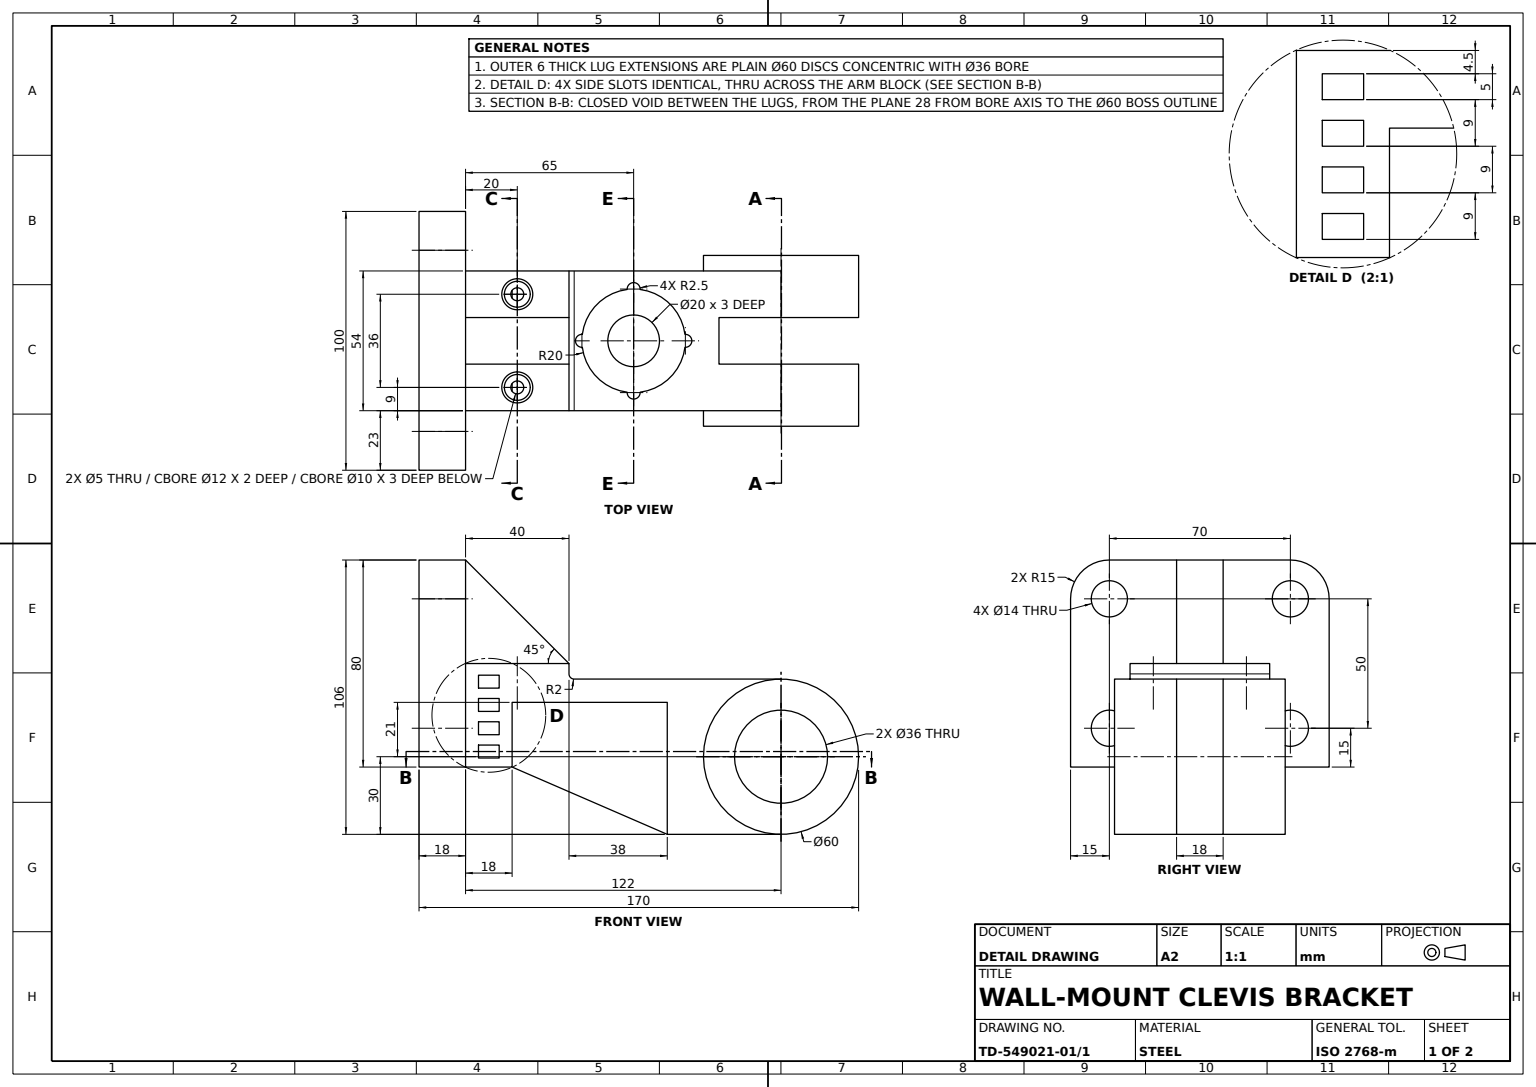
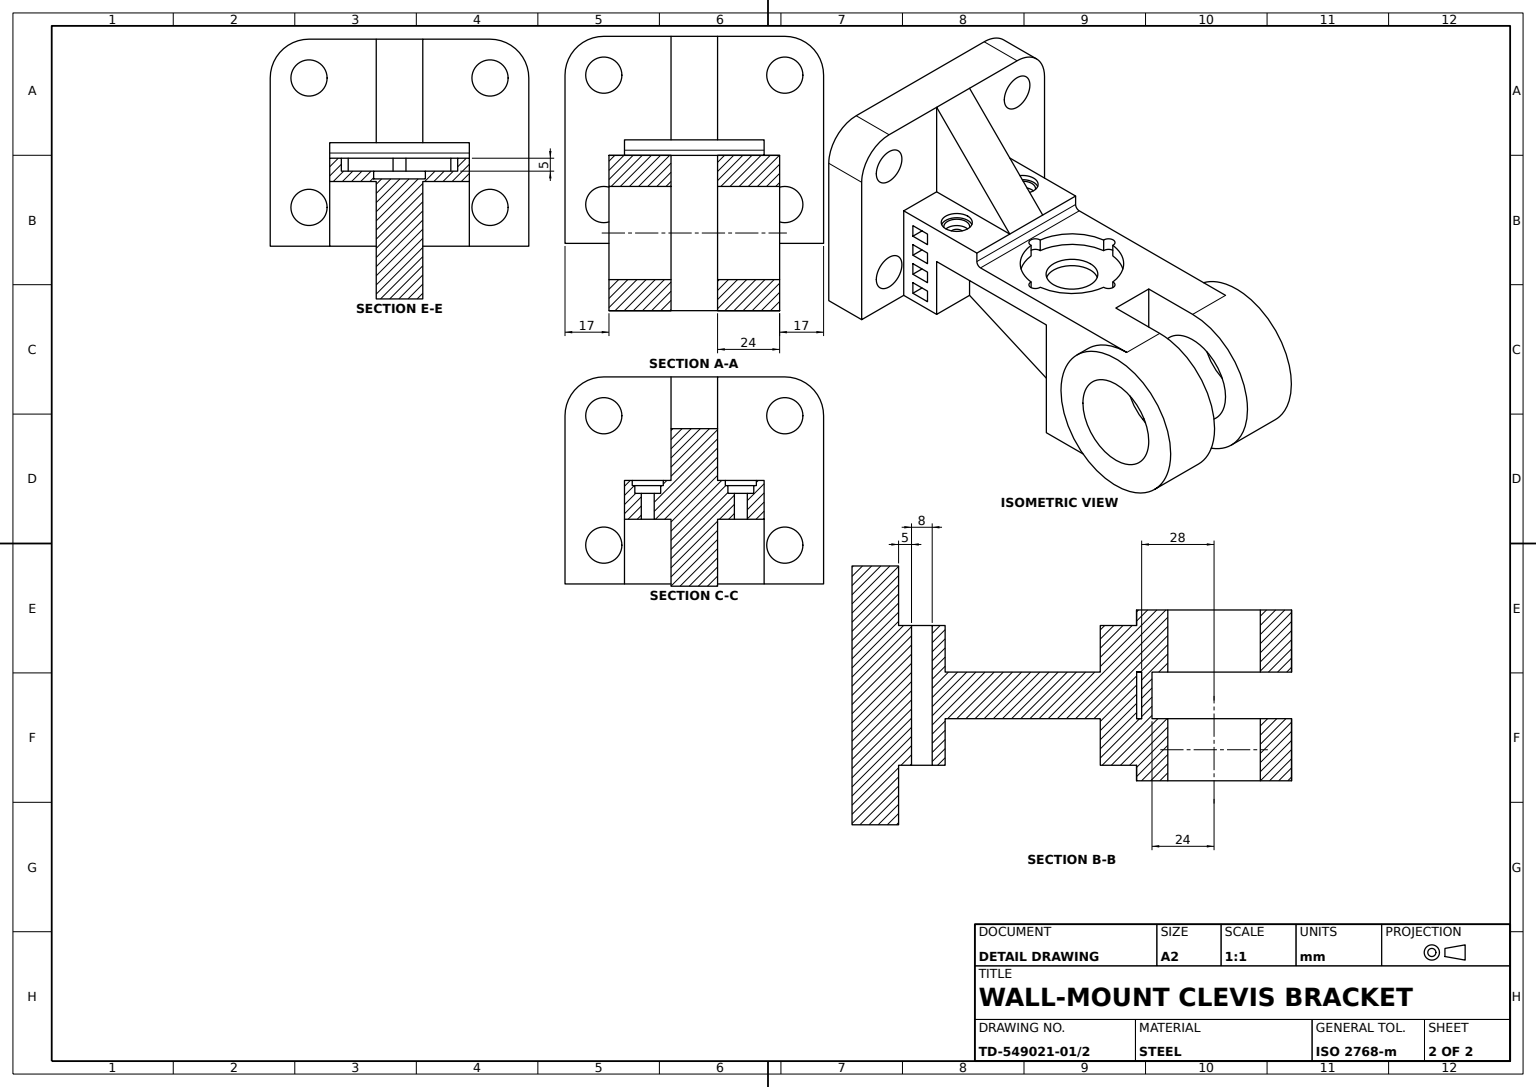
from build123d import *
from build123d.topology import SkipClean

# Parameters (mm, degrees)
MOUNTING_PLATE_SKETCH_R      = 9
MOUNTING_PLATE_DEPTH         = 18
ARM_BLOCK_SKETCH_W           = 18
ARM_BLOCK_SKETCH_H           = 54
ARM_BLOCK_DEPTH              = 40
PLATE_START                  = -18
PLATE_CORNER_BOSSES_SKETCH_R = 7
PLATE_CORNER_BOSSES_DEPTH    = 18
ARM_EXTENSION_SKETCH_W       = 40
ARM_EXTENSION_SKETCH_H       = 54
ARM_EXTENSION_DEPTH          = 15
UPPER_SUPPORT_RIB_REACH      = 88.394
UPPER_RIB_SKETCH_WALL_W      = 231.357431026
UPPER_RIB_SKETCH_WALL_H      = 18
CLEVIS_ARM_DEPTH             = 54
SKETCH7_4_R                  = 30
SKETCH7_4_R_2                = 18
CLEVIS_FACE_1_DEPTH          = 6
SKETCH7_5_R                  = 30
SKETCH7_5_R_2                = 18
CLEVIS_LUG_1_DEPTH           = 18
CLEVIS_START                 = -36
SKETCH7_6_R                  = 30
SKETCH7_6_R_2                = 18
CLEVIS_LUG_2_DEPTH           = 18
CLEVIS_START_2               = -54
SKETCH7_7_R                  = 30
SKETCH7_7_R_2                = 18
CLEVIS_FACE_2_DEPTH          = 6
CLEVIS_PIN_BORE_SKETCH_W     = 24
CLEVIS_PIN_BORE_SKETCH_H     = 18
CLEVIS_PIN_BORE_24_DEPTH     = 188.082869339
LOWER_SUPPORT_RIB_REACH      = 191.093
LOWER_RIB_SKETCH_WALL_W      = 445.576270742
LOWER_RIB_SKETCH_WALL_H      = 18
CLEVIS_WEB_PAD_SKETCH_W      = 4
CLEVIS_WEB_PAD_SKETCH_H      = 18
CLEVIS_WEB_PAD_DEPTH         = 60
ARM_BLOCK_HOLES_SKETCH_R     = 2.5
ARM_BLOCK_HOLES_DEPTH        = 15
COUNTERBORE_10_SKETCH_R      = 5
COUNTERBORE_10_DEPTH         = 5
SPOTFACE_12_SKETCH_R         = 6
SPOTFACE_12_DEPTH            = 2
SIDE_SLOTS_4X_SKETCH_W       = 8
SIDE_SLOTS_4X_SKETCH_H       = 5
SIDE_SLOTS_4X_DEPTH          = 198.952014387
KEYED_RECESS_SKETCH_R        = 10
KEYED_RECESS_DEPTH           = 5
RECESS_BORE_20_SKETCH_R      = 10
RECESS_BORE_20_DEPTH         = 8
ARM_EDGE_FILLET_R2_R         = 2


with BuildPart() as part:
    # Mounting Plate Sketch → Mounting Plate (new body)
    with BuildSketch(Plane(origin=(0, 0, 0), x_dir=(0, 0, -1), z_dir=(1, 0, 0))):
        with BuildLine():
            Line((-50, -40), (50, -40))
            Line((50, -40), (50, 25))
            ThreePointArc((50, 25), (45.606601718, 35.606601718), (35, 40))
            Line((35, 40), (-35, 40))
            ThreePointArc((-35, 40), (-45.606601718, 35.606601718), (-50, 25))
            Line((-50, 25), (-50, -40))
        make_face()
        with Locations((-35, 25)):
            Circle(MOUNTING_PLATE_SKETCH_R, mode=Mode.SUBTRACT)
        with Locations((35, 25)):
            Circle(MOUNTING_PLATE_SKETCH_R, mode=Mode.SUBTRACT)
        with Locations((-35, -25)):
            Circle(MOUNTING_PLATE_SKETCH_R, mode=Mode.SUBTRACT)
        with Locations((35, -25)):
            Circle(MOUNTING_PLATE_SKETCH_R, mode=Mode.SUBTRACT)
    extrude(amount=MOUNTING_PLATE_DEPTH)

    # Arm Block Sketch → Arm Block (add)
    with BuildSketch(Plane.XZ.offset(40)):
        with Locations((27, 0)):
            Rectangle(ARM_BLOCK_SKETCH_W, ARM_BLOCK_SKETCH_H)
    extrude(amount=-ARM_BLOCK_DEPTH)

    # Plate Corner Bosses Sketch → Plate Corner Bosses (add)
    with BuildSketch(Plane(origin=(18, 0, 0), x_dir=(0, 0, -1), z_dir=(1, 0, 0)).offset(PLATE_START)):
        with BuildLine():
            Line((-35, 40), (35, 40))
            ThreePointArc((35, 40), (45.606601718, 35.606601718), (50, 25))
            Line((50, 25), (50, -40))
            Line((50, -40), (-50, -40))
            Line((-50, -40), (-50, 25))
            ThreePointArc((-50, 25), (-45.606601718, 35.606601718), (-35, 40))
        make_face()
        with Locations((-35, 25)):
            Circle(PLATE_CORNER_BOSSES_SKETCH_R, mode=Mode.SUBTRACT)
        with Locations((35, 25)):
            Circle(PLATE_CORNER_BOSSES_SKETCH_R, mode=Mode.SUBTRACT)
        with Locations((35, -25)):
            Circle(PLATE_CORNER_BOSSES_SKETCH_R, mode=Mode.SUBTRACT)
        with Locations((-35, -25)):
            Circle(PLATE_CORNER_BOSSES_SKETCH_R, mode=Mode.SUBTRACT)
    extrude(amount=PLATE_CORNER_BOSSES_DEPTH)

    # Arm Extension Sketch → Arm Extension (add)
    with BuildSketch(Plane(origin=(0, 0, 0), x_dir=(1, 0, 0), z_dir=(0, 1, 0))):
        with Locations((38, 0)):
            Rectangle(ARM_EXTENSION_SKETCH_W, ARM_EXTENSION_SKETCH_H)
    extrude(amount=-ARM_EXTENSION_DEPTH)

    # Upper Rib Sketch wall → Upper Support Rib (add, up to next)
    with BuildSketch(Plane(origin=(38, 20, 0), x_dir=(0.707106781187, -0.707106781187, 0), z_dir=(0.707106781187, 0.707106781187, 0)), mode=Mode.PRIVATE) as upper_support_rib_sk1:
        Rectangle(UPPER_RIB_SKETCH_WALL_W, UPPER_RIB_SKETCH_WALL_H)
    upper_support_rib_tool1 = extrude(upper_support_rib_sk1.sketch, amount=-UPPER_SUPPORT_RIB_REACH, mode=Mode.PRIVATE) - part.part
    add(upper_support_rib_tool1.solids().sort_by_distance((38, 20, 0))[0])

    # Clevis Arm Profile Sketch → Clevis Arm (add)
    with BuildSketch(Plane.XY.offset(27)):
        with BuildLine():
            ThreePointArc((140, -66), (110, -36), (140, -6))
            Line((140, -6), (58, -6))
            Line((58, -6), (58, -15))
            Line((58, -15), (96, -15))
            Line((96, -15), (96, -66))
            Line((96, -66), (140, -66))
        make_face()
    extrude(amount=-CLEVIS_ARM_DEPTH)



with BuildPart() as body_2:
    # Sketch7_4 → Clevis Face 1 (new body)
    with BuildSketch(Plane.XY.offset(27)):
        with Locations((140, -36)):
            Circle(SKETCH7_4_R)
        with Locations((140, -36)):
            Circle(SKETCH7_4_R_2, mode=Mode.SUBTRACT)
    extrude(amount=CLEVIS_FACE_1_DEPTH)


with BuildPart() as part_1:
    with SkipClean():  # the faces are left unmerged after this step: merging them gives an invalid solid
        add(part.part)

        add(body_2.part)  # Clevis Lug 1 merges body 2
        # Sketch7_5 → Clevis Lug 1 (add)
        with BuildSketch(Plane.XY.offset(27)):
            with Locations((140, -36)):
                Circle(SKETCH7_5_R)
            with Locations((140, -36)):
                Circle(SKETCH7_5_R_2, mode=Mode.SUBTRACT)
        extrude(amount=-CLEVIS_LUG_1_DEPTH)

    # Sketch7_6 → Clevis Lug 2 (add)
    with SkipClean():  # the faces are left unmerged after this step: merging them gives an invalid solid
        with BuildSketch(Plane.XY.offset(27).offset(CLEVIS_START)):
            with Locations((140, -36)):
                Circle(SKETCH7_6_R)
            with Locations((140, -36)):
                Circle(SKETCH7_6_R_2, mode=Mode.SUBTRACT)
        extrude(amount=-CLEVIS_LUG_2_DEPTH)

    # Sketch7_7 → Clevis Face 2 (add)
    with SkipClean():  # the faces are left unmerged after this step: merging them gives an invalid solid
        with BuildSketch(Plane.XY.offset(27).offset(CLEVIS_START_2)):
            with Locations((140, -36)):
                Circle(SKETCH7_7_R)
            with Locations((140, -36)):
                Circle(SKETCH7_7_R_2, mode=Mode.SUBTRACT)
        extrude(amount=-CLEVIS_FACE_2_DEPTH)

    # Clevis Pin Bore Sketch → Clevis Pin Bore _24 (cut, through all)
    with SkipClean():  # the faces are left unmerged after this step: merging them gives an invalid solid
        with BuildSketch(Plane(origin=(0, -6, 0), x_dir=(1, 0, 0), z_dir=(0, 1, 0))):
            with Locations((128, 0)):
                Rectangle(CLEVIS_PIN_BORE_SKETCH_W, CLEVIS_PIN_BORE_SKETCH_H)
        extrude(amount=-CLEVIS_PIN_BORE_24_DEPTH, mode=Mode.SUBTRACT)

    # Lower Rib Sketch wall → Lower Support Rib (add, up to next)
    with BuildSketch(Plane(origin=(66, -53, 0), x_dir=(0.91755562531, -0.397607437634, 0), z_dir=(0.397607437634, 0.91755562531, 0)), mode=Mode.PRIVATE) as lower_support_rib_sk1:
        Rectangle(LOWER_RIB_SKETCH_WALL_W, LOWER_RIB_SKETCH_WALL_H)
    lower_support_rib_tool1 = extrude(lower_support_rib_sk1.sketch, amount=LOWER_SUPPORT_RIB_REACH, mode=Mode.PRIVATE) - part_1.part
    add(lower_support_rib_tool1.solids().sort_by_distance((66, -53, 0))[0])

    # Clevis Web Pad Sketch → Clevis Web Pad (add)
    with SkipClean():  # the faces are left unmerged after this step: merging them gives an invalid solid
        with BuildSketch(Plane(origin=(0, -6, 0), x_dir=(1, 0, 0), z_dir=(0, 1, 0))):
            with Locations((114, 0)):
                Rectangle(CLEVIS_WEB_PAD_SKETCH_W, CLEVIS_WEB_PAD_SKETCH_H)
        extrude(amount=-CLEVIS_WEB_PAD_DEPTH)

    # Arm Block Holes Sketch → Arm Block Holes (cut)
    with SkipClean():  # the faces are left unmerged after this step: merging them gives an invalid solid
        with BuildSketch(Plane(origin=(0, 0, 0), x_dir=(1, 0, 0), z_dir=(0, 1, 0))):
            with Locations(Location((38, 18, 0), (0, 0, 270))):
                Circle(ARM_BLOCK_HOLES_SKETCH_R)
            with Locations(Location((38, -18, 0), (0, 0, 270))):
                Circle(ARM_BLOCK_HOLES_SKETCH_R)
        extrude(amount=-ARM_BLOCK_HOLES_DEPTH, mode=Mode.SUBTRACT)

    # Counterbore _10 Sketch → Counterbore _10 (cut)
    with SkipClean():  # the faces are left unmerged after this step: merging them gives an invalid solid
        with BuildSketch(Plane(origin=(0, 0, 0), x_dir=(1, 0, 0), z_dir=(0, 1, 0))):
            with Locations(Location((38, 18, 0), (0, 0, 270))):
                Circle(COUNTERBORE_10_SKETCH_R)
            with Locations(Location((38, -18, 0), (0, 0, 270))):
                Circle(COUNTERBORE_10_SKETCH_R)
        extrude(amount=-COUNTERBORE_10_DEPTH, mode=Mode.SUBTRACT)

    # Spotface _12 Sketch → Spotface _12 (cut)
    with SkipClean():  # the faces are left unmerged after this step: merging them gives an invalid solid
        with BuildSketch(Plane(origin=(0, 0, 0), x_dir=(1, 0, 0), z_dir=(0, 1, 0))):
            with Locations(Location((38, 18, 0), (0, 0, 270))):
                Circle(SPOTFACE_12_SKETCH_R)
            with Locations(Location((38, -18, 0), (0, 0, 270))):
                Circle(SPOTFACE_12_SKETCH_R)
        extrude(amount=-SPOTFACE_12_DEPTH, mode=Mode.SUBTRACT)

    # Side Slots 4x Sketch → Side Slots 4x (cut, through all)
    with SkipClean():  # the faces are left unmerged after this step: merging them gives an invalid solid
        with BuildSketch(Plane.XY.offset(27)):
            with Locations((27, -7)):
                Rectangle(SIDE_SLOTS_4X_SKETCH_W, SIDE_SLOTS_4X_SKETCH_H)
            with Locations((27, -16)):
                Rectangle(SIDE_SLOTS_4X_SKETCH_W, SIDE_SLOTS_4X_SKETCH_H)
            with Locations((27, -25)):
                Rectangle(SIDE_SLOTS_4X_SKETCH_W, SIDE_SLOTS_4X_SKETCH_H)
            with Locations((27, -34)):
                Rectangle(SIDE_SLOTS_4X_SKETCH_W, SIDE_SLOTS_4X_SKETCH_H)
        extrude(amount=-SIDE_SLOTS_4X_DEPTH, mode=Mode.SUBTRACT)

    # Keyed Recess Sketch → Keyed Recess (cut)
    with SkipClean():  # the faces are left unmerged after this step: merging them gives an invalid solid
        with BuildSketch(Plane(origin=(0, -6, 0), x_dir=(1, 0, 0), z_dir=(0, 1, 0))):
            with BuildLine():
                ThreePointArc((63.15625, -2.49511241), (68.857864376, -14.142135624), (80.50488759, -19.84375))
                ThreePointArc((80.50488759, -19.84375), (83, -22.5), (85.49511241, -19.84375))
                ThreePointArc((85.49511241, -19.84375), (97.142135624, -14.142135624), (102.84375, -2.49511241))
                ThreePointArc((102.84375, -2.49511241), (105.5, 0), (102.84375, 2.49511241))
                ThreePointArc((102.84375, 2.49511241), (97.142135624, 14.142135624), (85.49511241, 19.84375))
                ThreePointArc((85.49511241, 19.84375), (83, 22.5), (80.50488759, 19.84375))
                ThreePointArc((80.50488759, 19.84375), (68.857864376, 14.142135624), (63.15625, 2.49511241))
                ThreePointArc((63.15625, 2.49511241), (60.5, 0), (63.15625, -2.49511241))
            make_face()
            with Locations(Location((83, 0, 0), (0, 0, 270))):
                Circle(KEYED_RECESS_SKETCH_R, mode=Mode.SUBTRACT)
        extrude(amount=-KEYED_RECESS_DEPTH, mode=Mode.SUBTRACT)

    # Recess Bore _20 Sketch → Recess Bore _20 (cut)
    with SkipClean():  # the faces are left unmerged after this step: merging them gives an invalid solid
        with BuildSketch(Plane(origin=(0, -6, 0), x_dir=(1, 0, 0), z_dir=(0, 1, 0))):
            with Locations(Location((83, 0, 0), (0, 0, 270))):
                Circle(RECESS_BORE_20_SKETCH_R)
        extrude(amount=-RECESS_BORE_20_DEPTH, mode=Mode.SUBTRACT)

    # Arm Edge Fillet R2
    arm_edge_fillet_r2_edges = [part_1.edges().sort_by_distance(p)[0] for p in [
        (58, -6, 0),
    ]]
    fillet(arm_edge_fillet_r2_edges, radius=ARM_EDGE_FILLET_R2_R)


solid = part_1.part
